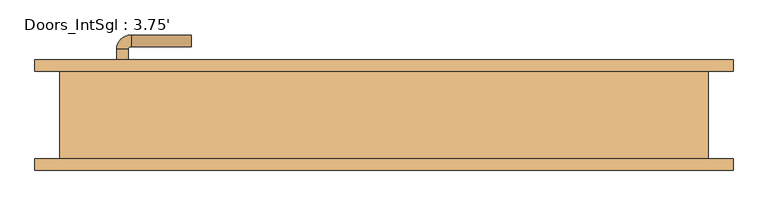
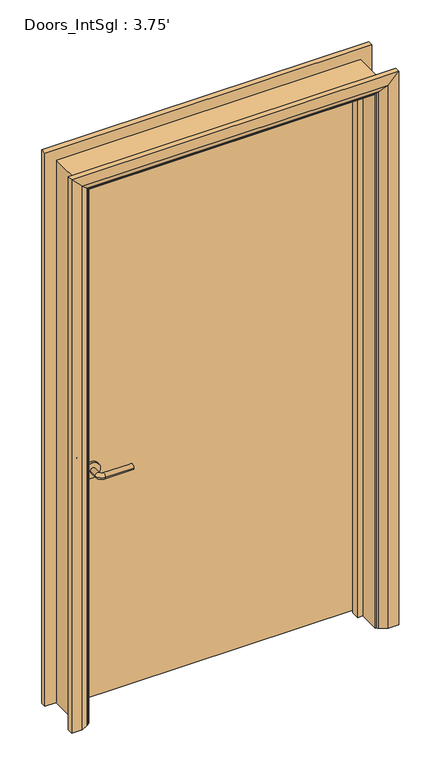
"""IFC4 building model written with IfcOpenShell, lengths in millimetres: door geometry, Doors_IntSgl : 3.75'."""

from ifc_helpers import new_model, si_unit, point, frame, frame_2d, origin, place, context, project, spatial, polyline, circle_curve, ellipse_curve, trimmed, segment, composite_curve, outline, extrude, faceted_brep, source, transform, mapped, element, save
from ifc_brep_helpers import plane_surface, cylinder_surface, revolved_surface, advanced_brep


def doors_intsgl_3_75_e7c258cb(model_context):
    return source(origin(), model_context, "Body", "SolidModel", [
        advanced_brep(
        [(-464.5, 30.2, 900.0), (-444.5, 30.2, 900.0), (-444.5, 0.2, 900.0), (-464.5, 0.2, 900.0), (-439.5, -4.8, 900.0), (-439.5, -24.8, 900.0), (-334.5, -24.8, 900.0), (-334.5, -4.8, 900.0)],
        [
            (0, 1, circle_curve(frame((-454.5, 30.2, 900.0), z_axis=(0.0, 1.0, 0.0), x_axis=(1.0, 0.0, 0.0)), 10.0)),
            (1, 0, circle_curve(frame((-454.5, 30.2, 900.0), z_axis=(0.0, 1.0, 0.0), x_axis=(1.0, 0.0, 0.0)), 10.0)),
            (1, 2),
            (2, 3, circle_curve(frame((-454.5, 0.2, 900.0), z_axis=(0.0, 1.0, 0.0), x_axis=(1.0, 0.0, 0.0)), 10.0)),
            (3, 0),
            (3, 2, circle_curve(frame((-454.5, 0.2, 900.0), z_axis=(0.0, 1.0, 0.0), x_axis=(1.0, 0.0, 0.0)), 10.0)),
            (4, 5, circle_curve(frame((-439.5, -14.8, 900.0), z_axis=(-1.0, 0.0, 0.0), x_axis=(0.0, 1.0, 0.0)), 10.0)),
            (5, 3, circle_curve(frame((-439.5, 0.2, 900.0), z_axis=(0.0, 0.0, -1.0), x_axis=(-1.0, 0.0, 0.0)), 25.0)),
            (2, 4, circle_curve(frame((-439.5, 0.2, 900.0), z_axis=(0.0, 0.0, 1.0), x_axis=(-1.0, 0.0, 0.0)), 5.0)),
            (5, 4, circle_curve(frame((-439.5, -14.8, 900.0), z_axis=(-1.0, 0.0, 0.0), x_axis=(0.0, 1.0, 0.0)), 10.0)),
            (6, 7, circle_curve(frame((-334.5, -14.8, 900.0), z_axis=(1.0, 0.0, 0.0), x_axis=(0.0, 1.0, 0.0)), 10.0)),
            (7, 6, circle_curve(frame((-334.5, -14.8, 900.0), z_axis=(1.0, 0.0, 0.0), x_axis=(0.0, 1.0, 0.0)), 10.0)),
            (4, 7),
            (6, 5),
        ],
        [
            plane_surface(frame((-454.5, 30.2, 900.0), z_axis=(0.0, 1.0, 0.0), x_axis=(0.0, 0.0, 1.0))),
            cylinder_surface(frame((-454.5, 30.2, 900.0), z_axis=(0.0, 1.0, 0.0), x_axis=(1.0, 0.0, 0.0)), 10.0),
            revolved_surface(trimmed(ellipse_curve(frame((-454.5, 0.2, 900.0), z_axis=(0.0, -1.0, 0.0), x_axis=(1.0, 0.0, 0.0)), 10.0, 10.0), [point((-464.5, 0.2, 900.0))], [point((-444.5, 0.2, 900.0))], True, "CARTESIAN"), (-439.5, 0.2, 900.0), (0.0, 0.0, -1.0)),
            revolved_surface(trimmed(ellipse_curve(frame((-454.5, 0.2, 900.0), z_axis=(0.0, -1.0, 0.0), x_axis=(1.0, 0.0, 0.0)), 10.0, 10.0), [point((-444.5, 0.2, 900.0))], [point((-464.5, 0.2, 900.0))], True, "CARTESIAN"), (-439.5, 0.2, 900.0), (0.0, 0.0, -1.0)),
            plane_surface(frame((-334.5, -14.8, 900.0), z_axis=(1.0, 0.0, 0.0), x_axis=(0.0, 0.0, 1.0))),
            cylinder_surface(frame((-439.5, -14.8, 900.0), z_axis=(-1.0, 0.0, 0.0), x_axis=(0.0, 1.0, 0.0)), 10.0),
        ],
        [
            (0, [[1, 2]]),
            (1, [[3, 4, 5, -2]]),
            (1, [[-5, 6, -3, -1]]),
            (2, [[7, 8, -4, 9]]),
            (3, [[10, -9, -6, -8]]),
            (4, [[11, 12]]),
            (5, [[13, -11, 14, -7]]),
            (5, [[-14, -12, -13, -10]]),
        ],
    ),
        extrude(outline(composite_curve([segment(trimmed(circle_curve(frame_2d((900.0, -457.0)), 30.0), [point((900.0, -487.0))], [point((900.0, -427.0))], False, "CARTESIAN"), True, "CONTINUOUS"), segment(trimmed(circle_curve(frame_2d((900.0, -457.0)), 30.0), [point((900.0, -427.0))], [point((900.0, -487.0))], False, "CARTESIAN"), True, "CONTINUOUS")], self_intersect=False)), frame((0.0, 30.2, 0.0), z_axis=(0.0, 1.0, 0.0), x_axis=(0.0, 0.0, 1.0)), (0.0, 0.0, 1.0), 8.0),
        advanced_brep(
        [(-464.5, 84.2, 900.0), (-444.5, 84.2, 900.0), (-464.5, 114.2, 900.0), (-444.5, 114.2, 900.0), (-439.5, 119.2, 900.0), (-439.5, 139.2, 900.0), (-334.5, 139.2, 900.0), (-334.5, 119.2, 900.0)],
        [
            (0, 1, circle_curve(frame((-454.5, 84.2, 900.0), z_axis=(0.0, -1.0, 0.0), x_axis=(1.0, 0.0, 0.0)), 10.0)),
            (1, 0, circle_curve(frame((-454.5, 84.2, 900.0), z_axis=(0.0, -1.0, 0.0), x_axis=(1.0, 0.0, 0.0)), 10.0)),
            (0, 2),
            (2, 3, circle_curve(frame((-454.5, 114.2, 900.0), z_axis=(0.0, -1.0, 0.0), x_axis=(1.0, 0.0, 0.0)), 10.0)),
            (3, 1),
            (3, 2, circle_curve(frame((-454.5, 114.2, 900.0), z_axis=(0.0, -1.0, 0.0), x_axis=(1.0, 0.0, 0.0)), 10.0)),
            (4, 3, circle_curve(frame((-439.5, 114.2, 900.0), z_axis=(0.0, 0.0, 1.0), x_axis=(-1.0, 0.0, 0.0)), 5.0)),
            (2, 5, circle_curve(frame((-439.5, 114.2, 900.0), z_axis=(0.0, 0.0, -1.0), x_axis=(-1.0, 0.0, 0.0)), 25.0)),
            (5, 4, circle_curve(frame((-439.5, 129.2, 900.0), z_axis=(-1.0, 0.0, 0.0), x_axis=(0.0, -1.0, 0.0)), 10.0)),
            (4, 5, circle_curve(frame((-439.5, 129.2, 900.0), z_axis=(-1.0, 0.0, 0.0), x_axis=(0.0, -1.0, 0.0)), 10.0)),
            (6, 7, circle_curve(frame((-334.5, 129.2, 900.0), z_axis=(1.0, 0.0, 0.0), x_axis=(0.0, -1.0, 0.0)), 10.0)),
            (7, 6, circle_curve(frame((-334.5, 129.2, 900.0), z_axis=(1.0, 0.0, 0.0), x_axis=(0.0, -1.0, 0.0)), 10.0)),
            (5, 6),
            (7, 4),
        ],
        [
            plane_surface(frame((-454.5, 84.2, 900.0), z_axis=(0.0, -1.0, 0.0), x_axis=(0.0, 0.0, 1.0))),
            cylinder_surface(frame((-454.5, 84.2, 900.0), z_axis=(0.0, -1.0, 0.0), x_axis=(1.0, 0.0, 0.0)), 10.0),
            revolved_surface(trimmed(ellipse_curve(frame((-454.5, 114.2, 900.0), z_axis=(0.0, -1.0, 0.0), x_axis=(1.0, 0.0, 0.0)), 10.0, 10.0), [point((-464.5, 114.2, 900.0))], [point((-444.5, 114.2, 900.0))], True, "CARTESIAN"), (-439.5, 114.2, 900.0), (0.0, 0.0, -1.0)),
            revolved_surface(trimmed(ellipse_curve(frame((-454.5, 114.2, 900.0), z_axis=(0.0, -1.0, 0.0), x_axis=(1.0, 0.0, 0.0)), 10.0, 10.0), [point((-444.5, 114.2, 900.0))], [point((-464.5, 114.2, 900.0))], True, "CARTESIAN"), (-439.5, 114.2, 900.0), (0.0, 0.0, -1.0)),
            plane_surface(frame((-334.5, 129.2, 900.0), z_axis=(1.0, 0.0, 0.0), x_axis=(0.0, 0.0, 1.0))),
            cylinder_surface(frame((-439.5, 129.2, 900.0), z_axis=(-1.0, 0.0, 0.0), x_axis=(0.0, -1.0, 0.0)), 10.0),
        ],
        [
            (0, [[1, 2]]),
            (1, [[-1, 3, 4, 5]]),
            (1, [[-2, -5, 6, -3]]),
            (2, [[7, -4, 8, 9]]),
            (3, [[-8, -6, -7, 10]]),
            (4, [[11, 12]]),
            (5, [[-9, 13, -12, 14]]),
            (5, [[-10, -14, -11, -13]]),
        ],
    ),
        extrude(outline(composite_curve([segment(trimmed(circle_curve(frame_2d((900.0, -457.0)), 30.0), [point((900.0, -487.0))], [point((900.0, -427.0))], False, "CARTESIAN"), True, "CONTINUOUS"), segment(trimmed(circle_curve(frame_2d((900.0, -457.0)), 30.0), [point((900.0, -427.0))], [point((900.0, -487.0))], False, "CARTESIAN"), True, "CONTINUOUS")], self_intersect=False)), frame((0.0, 76.2, 0.0), z_axis=(0.0, 1.0, 0.0), x_axis=(0.0, 0.0, 1.0)), (0.0, 0.0, 1.0), 8.0),
        extrude(outline(polyline([(529.5, 38.2), (-529.5, 38.2), (-529.5, 76.2), (529.5, 76.2), (529.5, 38.2)])), frame((0.0, 0.0, 8.0), z_axis=(0.0, 0.0, 1.0), x_axis=(1.0, 0.0, 0.0)), (0.0, 0.0, 1.0), 2083.6),
        advanced_brep(
        [(606.5, 96.2, 0.0), (606.5, 76.2, 0.0), (536.5, 76.2, 0.0), (540.5, 82.2, 0.0), (566.5, 96.2, 0.0), (606.5, 96.2, 2168.6), (606.5, 76.2, 2168.6), (-606.5, 76.2, 2168.6), (-606.5, 76.2, 0.0), (-536.5, 76.2, 0.0), (-536.5, 76.2, 2098.6), (536.5, 76.2, 2098.6), (540.5, 82.2, 2102.6), (566.5, 96.2, 2128.6), (-566.5, 96.2, 2128.6), (-566.5, 96.2, 0.0), (-606.5, 96.2, 0.0), (-606.5, 96.2, 2168.6), (-540.5, 82.2, 0.0), (-540.5, 82.2, 2102.6)],
        [
            (0, 1),
            (1, 2),
            (2, 3, circle_curve(frame((544.5, 75.2, 0.0), z_axis=(0.0, 0.0, -1.0), x_axis=(1.0, 0.0, 0.0)), 8.0622577)),
            (3, 4),
            (4, 0),
            (0, 5),
            (5, 6),
            (6, 1),
            (6, 7),
            (7, 8),
            (8, 9),
            (9, 10),
            (10, 11),
            (11, 2),
            (11, 12, ellipse_curve(frame((544.5, 75.2, 2106.6), z_axis=(0.7071067811865475, 0.0, -0.7071067811865475), x_axis=(-0.7071067811865474, 0.0, -0.7071067811865476)), 11.4017543, 8.0622577)),
            (12, 3),
            (12, 13),
            (13, 4),
            (13, 14),
            (14, 15),
            (15, 16),
            (16, 17),
            (17, 5),
            (7, 17),
            (16, 8),
            (15, 18),
            (18, 9, circle_curve(frame((-544.5, 75.2, 0.0), z_axis=(0.0, 0.0, -1.0), x_axis=(-1.0, 0.0, 0.0)), 8.0622577)),
            (19, 10, ellipse_curve(frame((-544.5, 75.2, 2106.6), z_axis=(-0.7071067811865475, 0.0, -0.7071067811865475), x_axis=(-0.7071067811865474, 0.0, 0.7071067811865476)), 11.4017543, 8.0622577)),
            (18, 19),
            (14, 19),
            (19, 12),
        ],
        [
            plane_surface(frame((536.5, 76.2, 0.0), z_axis=(0.0, 0.0, -1.0), x_axis=(0.0, -1.0, 0.0))),
            plane_surface(frame((606.5, 96.2, 0.0), z_axis=(1.0, 0.0, 0.0), x_axis=(0.0, 0.0, 1.0))),
            plane_surface(frame((606.5, 76.2, 0.0), z_axis=(0.0, -1.0, 0.0), x_axis=(0.0, 0.0, 1.0))),
            cylinder_surface(frame((544.5, 75.2, 0.0), z_axis=(0.0, 0.0, -1.0), x_axis=(1.0, 0.0, 0.0)), 8.0622577),
            plane_surface(frame((540.5, 82.2, 0.0), z_axis=(-0.4740998230350126, 0.880471099922178, 0.0), x_axis=(0.0, 0.0, 1.0))),
            plane_surface(frame((566.5, 96.2, 0.0), z_axis=(0.0, 1.0, 0.0), x_axis=(0.0, 0.0, 1.0))),
            plane_surface(frame((-606.5, 96.2, 2168.6), z_axis=(-1.0, 0.0, 0.0), x_axis=(0.0, 0.0, -1.0))),
            plane_surface(frame((-536.5, 76.2, 0.0), z_axis=(0.0, 0.0, -1.0), x_axis=(0.0, -1.0, 0.0))),
            cylinder_surface(frame((-544.5, 75.2, 2098.6), z_axis=(0.0, 0.0, 1.0), x_axis=(-1.0, 0.0, 0.0)), 8.0622577),
            plane_surface(frame((-540.5, 82.2, 2102.6), z_axis=(0.47409982303501824, 0.8804710999221749, 0.0), x_axis=(0.0, 0.0, -1.0))),
            plane_surface(frame((606.5, 96.2, 2168.6), z_axis=(0.0, 0.0, 1.0), x_axis=(-1.0, 0.0, 0.0))),
            cylinder_surface(frame((536.5, 75.2, 2106.6), z_axis=(1.0, 0.0, 0.0), x_axis=(0.0, 0.0, 1.0)), 8.0622577),
            plane_surface(frame((540.5, 82.2, 2102.6), z_axis=(0.0, 0.8804710999221764, -0.4740998230350154), x_axis=(-1.0, 0.0, 0.0))),
        ],
        [
            (0, [[1, 2, 3, 4, 5]]),
            (1, [[-1, 6, 7, 8]]),
            (2, [[-2, -8, 9, 10, 11, 12, 13, 14]]),
            (3, [[-3, -14, 15, 16]]),
            (4, [[-4, -16, 17, 18]]),
            (5, [[-5, -18, 19, 20, 21, 22, 23, -6]]),
            (6, [[24, -22, 25, -10]]),
            (7, [[-21, 26, 27, -11, -25]]),
            (8, [[28, -12, -27, 29]]),
            (9, [[30, -29, -26, -20]]),
            (10, [[-7, -23, -24, -9]]),
            (11, [[-15, -13, -28, 31]]),
            (12, [[-17, -31, -30, -19]]),
        ],
    ),
        extrude(outline(polyline([(0.0, -531.5), (0.0, -512.5), (2074.6, -512.5), (2074.6, 512.5), (0.0, 512.5), (0.0, 531.5), (2093.6, 531.5), (2093.6, -531.5), (0.0, -531.5)])), frame((0.0, 4.2, 0.0), z_axis=(0.0, 1.0, 0.0), x_axis=(0.0, 0.0, 1.0)), (0.0, 0.0, 1.0), 32.0),
        advanced_brep(
        [(-606.5, -96.2, 0.0), (-606.5, -76.2, 0.0), (-536.5, -76.2, 0.0), (-540.5, -82.2, 0.0), (-566.5, -96.2, 0.0), (-606.5, -96.2, 2168.6), (-606.5, -76.2, 2168.6), (-536.5, -76.2, 2098.6), (-540.5, -82.2, 2102.6), (-566.5, -96.2, 2128.6), (606.5, -96.2, 0.0), (566.5, -96.2, 0.0), (540.5, -82.2, 0.0), (536.5, -76.2, 0.0), (606.5, -76.2, 0.0), (606.5, -96.2, 2168.6), (566.5, -96.2, 2128.6), (540.5, -82.2, 2102.6), (536.5, -76.2, 2098.6), (606.5, -76.2, 2168.6)],
        [
            (0, 1),
            (1, 2),
            (2, 3, circle_curve(frame((-544.5, -75.2, 0.0), z_axis=(0.0, 0.0, -1.0), x_axis=(-1.0, 0.0, 0.0)), 8.0622577)),
            (3, 4),
            (4, 0),
            (0, 5),
            (5, 6),
            (6, 1),
            (6, 7),
            (7, 2),
            (7, 8, ellipse_curve(frame((-544.5, -75.2, 2106.6), z_axis=(-0.7071067811865475, 0.0, -0.7071067811865475), x_axis=(0.7071067811865474, 0.0, -0.7071067811865476)), 11.4017543, 8.0622577)),
            (8, 3),
            (8, 9),
            (9, 4),
            (9, 5),
            (10, 11),
            (11, 12),
            (12, 13, circle_curve(frame((544.5, -75.2, 0.0), z_axis=(0.0, 0.0, -1.0), x_axis=(1.0, 0.0, 0.0)), 8.0622577)),
            (13, 14),
            (14, 10),
            (15, 16),
            (16, 11),
            (10, 15),
            (16, 17),
            (17, 12),
            (17, 18, ellipse_curve(frame((544.5, -75.2, 2106.6), z_axis=(0.7071067811865475, 0.0, -0.7071067811865475), x_axis=(0.7071067811865474, 0.0, 0.7071067811865476)), 11.4017543, 8.0622577)),
            (18, 13),
            (18, 19),
            (19, 14),
            (19, 15),
            (5, 15),
            (19, 6),
            (18, 7),
            (17, 8),
            (16, 9),
        ],
        [
            plane_surface(frame((-536.5, -149.0010989, 0.0), z_axis=(0.0, 0.0, -1.0), x_axis=(1.0, 0.0, 0.0))),
            plane_surface(frame((-606.5, -96.2, 0.0), z_axis=(-1.0, 0.0, 0.0), x_axis=(0.0, 0.0, 1.0))),
            plane_surface(frame((-606.5, -76.2, 0.0), z_axis=(0.0, 1.0, 0.0), x_axis=(0.0, 0.0, 1.0))),
            cylinder_surface(frame((-544.5, -75.2, 0.0), z_axis=(0.0, 0.0, -1.0), x_axis=(-1.0, 0.0, 0.0)), 8.0622577),
            plane_surface(frame((-540.5, -82.2, 0.0), z_axis=(0.4740998230350183, -0.8804710999221749, 0.0), x_axis=(0.0, 0.0, 1.0))),
            plane_surface(frame((-566.5, -96.2, 0.0), z_axis=(0.0, -1.0, 0.0), x_axis=(0.0, 0.0, 1.0))),
            plane_surface(frame((536.5, -149.0010989, 0.0), z_axis=(0.0, 0.0, -1.0), x_axis=(-1.0, 0.0, 0.0))),
            plane_surface(frame((566.5, -96.2, 2128.6), z_axis=(0.0, -1.0, 0.0), x_axis=(0.0, 0.0, -1.0))),
            plane_surface(frame((540.5, -82.2, 2102.6), z_axis=(-0.4740998230350183, -0.8804710999221749, 0.0), x_axis=(0.0, 0.0, -1.0))),
            cylinder_surface(frame((544.5, -75.2, 2098.6), z_axis=(0.0, 0.0, 1.0), x_axis=(1.0, 0.0, 0.0)), 8.0622577),
            plane_surface(frame((606.5, -76.2, 2168.6), z_axis=(0.0, 1.0, 0.0), x_axis=(0.0, 0.0, -1.0))),
            plane_surface(frame((606.5, -96.2, 2168.6), z_axis=(1.0, 0.0, 0.0), x_axis=(0.0, 0.0, -1.0))),
            plane_surface(frame((-606.5, -96.2, 2168.6), z_axis=(0.0, 0.0, 1.0), x_axis=(1.0, 0.0, 0.0))),
            plane_surface(frame((-606.5, -76.2, 2168.6), z_axis=(0.0, 1.0, 0.0), x_axis=(1.0, 0.0, 0.0))),
            cylinder_surface(frame((-536.5, -75.2, 2106.6), z_axis=(-1.0, 0.0, 0.0), x_axis=(0.0, 0.0, 1.0)), 8.0622577),
            plane_surface(frame((-540.5, -82.2, 2102.6), z_axis=(0.0, -0.8804710999221749, -0.4740998230350183), x_axis=(1.0, 0.0, 0.0))),
            plane_surface(frame((-566.5, -96.2, 2128.6), z_axis=(0.0, -1.0, 0.0), x_axis=(1.0, 0.0, 0.0))),
        ],
        [
            (0, [[1, 2, 3, 4, 5]]),
            (1, [[-1, 6, 7, 8]]),
            (2, [[-2, -8, 9, 10]]),
            (3, [[-3, -10, 11, 12]]),
            (4, [[-4, -12, 13, 14]]),
            (5, [[-5, -14, 15, -6]]),
            (6, [[16, 17, 18, 19, 20]]),
            (7, [[21, 22, -16, 23]]),
            (8, [[24, 25, -17, -22]]),
            (9, [[26, 27, -18, -25]]),
            (10, [[28, 29, -19, -27]]),
            (11, [[30, -23, -20, -29]]),
            (12, [[-7, 31, -30, 32]]),
            (13, [[-9, -32, -28, 33]]),
            (14, [[-11, -33, -26, 34]]),
            (15, [[-13, -34, -24, 35]]),
            (16, [[-15, -35, -21, -31]]),
        ],
    ),
        faceted_brep([(-531.5, 76.2, 0.0), (-531.5, -76.2, 0.0), (-563.5, -76.2, 0.0), (-563.5, 76.2, 0.0), (-531.5, 76.2, 2093.6), (-531.5, -76.2, 2093.6), (-563.5, -76.2, 2125.6), (-563.5, 76.2, 2125.6), (531.5, 76.2, 0.0), (563.5, 76.2, 0.0), (563.5, -76.2, 0.0), (531.5, -76.2, 0.0), (531.5, 76.2, 2093.6), (563.5, 76.2, 2125.6), (563.5, -76.2, 2125.6), (531.5, -76.2, 2093.6)], [[[0, 1, 2, 3]], [[1, 0, 4, 5]], [[2, 1, 5, 6]], [[3, 2, 6, 7]], [[0, 3, 7, 4]], [[8, 9, 10, 11]], [[12, 13, 9, 8]], [[13, 14, 10, 9]], [[14, 15, 11, 10]], [[15, 12, 8, 11]], [[5, 4, 12, 15]], [[6, 5, 15, 14]], [[7, 6, 14, 13]], [[4, 7, 13, 12]]]),
    ])


if __name__ == "__main__":
    model = new_model("IFC4")
    model_context = context("Model", 3, world=origin())
    ifc_project = project(units=[si_unit("LENGTHUNIT", "METRE", prefix="MILLI")], contexts=[model_context])
    site = spatial("IfcSite", under=ifc_project)
    building = spatial("IfcBuilding", under=site)
    placement = place(None, origin())
    doors_intsgl_3_75_shape = doors_intsgl_3_75_e7c258cb(model_context)
    element("IfcDoor", 1, ObjectType="Doors_IntSgl : 3.75'", at=placement, inside=building, context=model_context, shape_type="MappedRepresentation", body=[
        mapped(doors_intsgl_3_75_shape, transform((0.0, 0.0, 0.0), x_axis=(1.0, 0.0, 0.0), y_axis=(0.0, 1.0, 0.0), z_axis=(0.0, 0.0, 1.0))),
    ])
    save(model, "model.ifc")

# Revit data of these elements
# Type "Doors_IntSgl : 3.75'"
#   Type Mark = "58"
#   Type Comments = "Internal Single"
#   Operation = "SingleSwingRight"
#   Manufacturer = "Revit"
#   Keynote = "L20"
#   Description = "Internal Single Door"
#   Analytic Construction = "Metal"
#   UnderCut = 8 mm
#   Tolerance = 2 mm
#   Thickness = 38 mm
#   Thermal Resistance (R) = 0.270117 (m²·K)/W
#   Structural Tolerance = 8 mm
#   StopDepth = 32 mm
#   Stop Thickness = 19 mm
#   Rough Width = 1143 mm
#   Rough Height = 2133.6 mm
#   Height to Top Lock Rail = 1000 mm
#   Heat Transfer Coefficient (U) = 3.7021 W/(m²·K)
#   Handle Z Distance = 900 mm
#   Handle X Distance = 75 mm
#   Frame Thickness = 32 mm
#   Door Panel Width = 1059 mm
#   Door Panel Thickness = 38 mm
#   Door Panel Offset = 0 mm
#   Height = 2133.6 mm
#   Width = 1143 mm
#   Door Panel Height = 2083.6 mm
#   Architrave Setback = 5 mm
#   Vis - Ironmongery = yes
#   Material Ironmongery = Door - Handle
#   Material Frame = Door - Frame/Mullion (1)
#   Material Door = Door - Panel
#   Material Architrave = Door - Architrave
#   Visual Light Transmittance = 0
#   Solar Heat Gain Coefficient = 0
#   Function = (empty or 0)
#   Wall Closure = (empty or 0)
# Element 1 (IfcDoor, "Doors_IntSgl : 3.75'")
#   Materials on its faces: "Door - Architrave", "Door - Handle", "Door - Frame/Mullion (1)", "Door - Panel"
# Materials
#   "Door - Handle": colour RGB 0 0 0, transparency 0, Keynote = "P21", Cost = 0
#   "Door - Frame/Mullion (1)": class "Wood", colour RGB 212 179 113, transparency 0, Keynote = "L20", Cost = 0
#   "Door - Panel": class "Wood", colour RGB 210 159 95, transparency 0, Keynote = "L20", Cost = 0
#   "Door - Architrave": class "Wood", colour RGB 154 90 5, transparency 0, Keynote = "P20", Cost = 0
